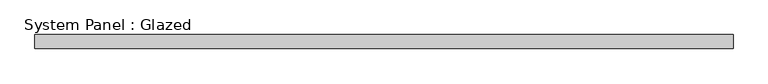
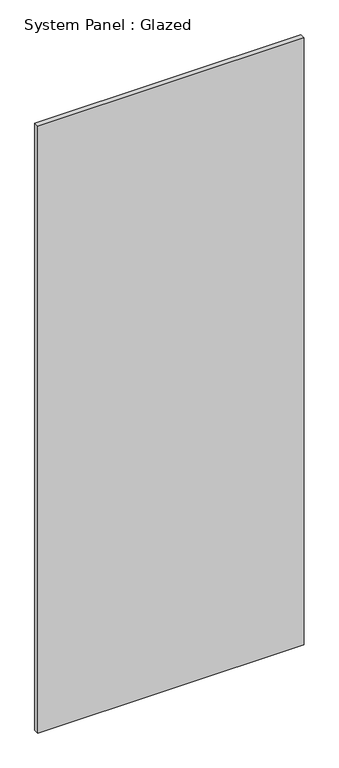
"""IFC4 building model written with IfcOpenShell, lengths in millimetres: plate geometry, System Panel : Glazed."""

from ifc_helpers import new_model, si_unit, origin, origin_with_axes, place, context, project, spatial, polyline, outline, extrude, source, transform, mapped, element, save


def system_panel_glazed_4b9268f2(model_context):
    return source(origin(), model_context, "Body", "SweptSolid", [
        extrude(outline(polyline([(622.3, 24.5), (-622.3, 24.5), (-622.3, 49.5), (622.3, 49.5), (622.3, 24.5)])), origin_with_axes(), (0.0, 0.0, 1.0), 3000.0),
    ])


if __name__ == "__main__":
    model = new_model("IFC4")
    model_context = context("Model", 3, world=origin())
    ifc_project = project(units=[si_unit("LENGTHUNIT", "METRE", prefix="MILLI")], contexts=[model_context])
    site = spatial("IfcSite", under=ifc_project)
    building = spatial("IfcBuilding", under=site)
    placement = place(None, origin())
    system_panel_glazed_shape = system_panel_glazed_4b9268f2(model_context)
    element("IfcPlate", 1, ObjectType="System Panel : Glazed", at=placement, inside=building, context=model_context, shape_type="MappedRepresentation", body=[
        mapped(system_panel_glazed_shape, transform((0.0, 0.0, 0.0), x_axis=(1.0, 0.0, 0.0), y_axis=(0.0, 1.0, 0.0), z_axis=(0.0, 0.0, 1.0))),
    ])
    save(model, "model.ifc")

# Revit data of these elements
# Type "System Panel : Glazed"
#   Keynote = "H11"
#   Construction Type Id = "GSP4R"
#   Analytic Construction = "1/8 in Pilkington single glazing"
#   Visual Light Transmittance = 0.9
#   Solar Heat Gain Coefficient = 0.86
#   Heat Transfer Coefficient (U) = 6.7069 W/(m²·K)
#   Define Thermal Properties by = 1
# Element 1 (IfcPlate, "System Panel : Glazed")
#   Materials on its faces: "Glass"
# Materials
#   "Glass": class "Glass", colour RGB 0 128 192, transparency 0.9, Description = "Soda Lime Glass", Cost = 0
